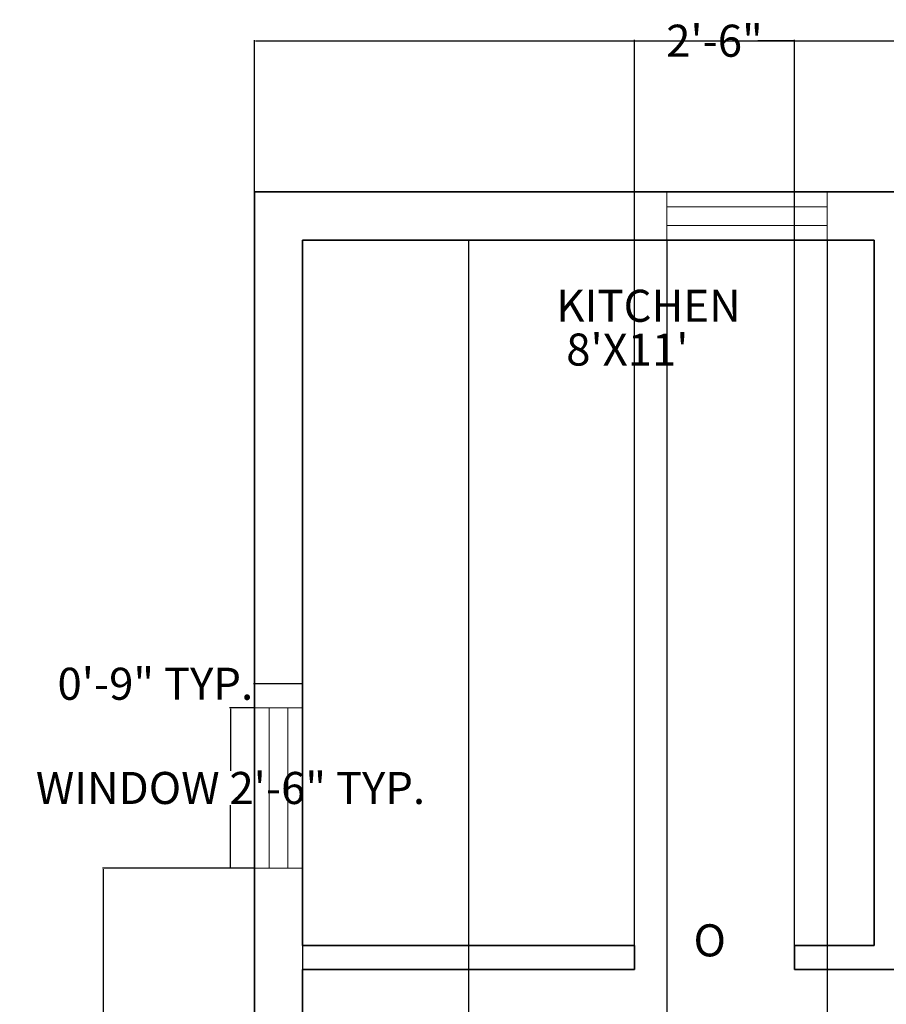
# Model space of a CAD drawing. Units: inches. Extents: x -26 to 575, y -18 to 513.
# Tile 10 of 28: x -26 to 136, y 324 to 508. Entities that reach past the tile are written whole.
import ezdxf

# ---------------------------------------------------------------- set-up
doc = ezdxf.new("R2010")
doc.units = ezdxf.units.IN
doc.header["$MEASUREMENT"] = 0
for name, color, linetype, lineweight in [('A-ANNO-DIMS', 2, 'Continuous', 18), ('A-ANNO-TEXT', 7, 'Continuous', 18), ('A-AREA-IDEN', 7, 'Continuous', 18), ('A-FLOR-CASE', 8, 'Continuous', 18), ('A-GLAZ', 4, 'Continuous', 18), ('A-WALL', 7, 'Continuous', 35)]:
    doc.layers.add(name, color=color, linetype=linetype, lineweight=lineweight)
doc.styles.get("Standard").update_dxf_attribs({"font": 'arial.ttf', "height": 6})
doc.dimstyles.get("Standard").update_dxf_attribs({"dimtxt": 6, "dimasz": 0.18, "dimexe": 0.18, "dimexo": 0.0625, "dimgap": 0.09, "dimtad": 0, "dimtih": 1, "dimtoh": 1, "dimzin": 0, "dimdsep": 46, "dimlunit": 3, "dimtxsty": 'Standard', "dimcen": 0.09, "dimadec": 0, "dimazin": 0, "dimtfac": 1, "dimtofl": 0, "dimtmove": 0, "dimatfit": 3, "dimfxl": 1, "dimtolj": 1, "dimtzin": 0, "dimarcsym": 0})

# ---------------------------------------------------------------- blocks, each defined once
blk = doc.blocks.new('*D1')
at = {"layer": 'A-ANNO-DIMS', "color": 0, "lineweight": -2, "transparency": 16777216}
for p, q in [((18.18, 475.57), (18.18, 503.94)), ((18.36, 503.76), (264.87, 503.76)), ((522, 503.76), (275.48, 503.76)), ((522.18, 475.57), (522.18, 503.94))]:
    blk.add_line(p, q, dxfattribs=at)
at = {"layer": 'A-ANNO-DIMS', "color": 0, "transparency": 16777216}
for points in [[(18.36, 503.79), (18.36, 503.73), (18.18, 503.76)], [(522, 503.79), (522, 503.73), (522.18, 503.76)]]:
    blk.add_solid(points, dxfattribs=at)
at = {"layer": 'Defpoints', "color": 0, "transparency": 16777216}
for p in [(522.18, 503.76), (18.18, 475.51), (522.18, 475.51)]:
    blk.add_point(p, dxfattribs=at)
at = {"layer": 'A-ANNO-DIMS', "color": 0, "transparency": 16777216, "insert": (270.18, 503.76), "char_height": 6, "attachment_point": 5}
blk.add_mtext("\\A1;42'", dxfattribs=at)
blk = doc.blocks.new('WINDOW-30IN')
for p, q in [((30, 9), (0, 9)), ((0, 9), (0, 0)), ((30, 0), (30, 9)), ((30, 6.25), (0, 6.25)), ((30, 0), (30, 4.5)), ((30, 2.75), (0, 2.75)), ((0, 0), (30, 0))]:
    blk.add_line(p, q)
blk = doc.blocks.new('*D18')
at = {"layer": 'A-ANNO-DIMS', "color": 0, "lineweight": -2, "transparency": 16777216}
for p, q in [((18.11, 378.99), (13.5, 378.99)), ((13.68, 378.81), (13.68, 367.18)), ((13.68, 349.17), (13.68, 360.79)), ((18.11, 348.99), (13.5, 348.99))]:
    blk.add_line(p, q, dxfattribs=at)
at = {"layer": 'A-ANNO-DIMS', "color": 0, "transparency": 16777216}
for points in [[(13.65, 378.81), (13.71, 378.81), (13.68, 378.99)], [(13.65, 349.17), (13.71, 349.17), (13.68, 348.99)]]:
    blk.add_solid(points, dxfattribs=at)
at = {"layer": 'Defpoints', "color": 0, "transparency": 16777216}
for p in [(18.18, 378.99), (13.68, 348.99), (18.18, 348.99)]:
    blk.add_point(p, dxfattribs=at)
at = {"layer": 'A-ANNO-DIMS', "color": 0, "transparency": 16777216, "insert": (13.68, 363.99), "char_height": 6, "attachment_point": 5}
blk.add_mtext('\\A1;WINDOW 2\'-6" TYP.', dxfattribs=at)
blk = doc.blocks.new('*D19')
at = {"layer": 'A-ANNO-DIMS', "color": 0, "lineweight": -2, "transparency": 16777216}
for p, q in [((18.18, 383.49), (18, 383.49)), ((18.18, 379.05), (18.18, 383.67)), ((27, 383.49), (18.36, 383.49)), ((27.18, 379.05), (27.18, 383.67))]:
    blk.add_line(p, q, dxfattribs=at)
at = {"layer": 'A-ANNO-DIMS', "color": 0, "transparency": 16777216}
for points in [[(18.36, 383.52), (18.36, 383.46), (18.18, 383.49)], [(27, 383.52), (27, 383.46), (27.18, 383.49)]]:
    blk.add_solid(points, dxfattribs=at)
at = {"layer": 'Defpoints', "color": 0, "transparency": 16777216}
for p in [(18.18, 383.49), (18.18, 378.99), (27.18, 378.99)]:
    blk.add_point(p, dxfattribs=at)
at = {"layer": 'A-ANNO-DIMS', "color": 0, "transparency": 16777216, "insert": (-0.38, 383.49), "char_height": 6, "attachment_point": 5}
blk.add_mtext('\\A1;0\'-9" TYP.', dxfattribs=at)
blk = doc.blocks.new('*D28')
at = {"layer": 'A-ANNO-DIMS', "color": 0, "lineweight": -2, "transparency": 16777216}
for p, q in [((58.22, 466.45), (58.22, -8.97)), ((95.35, 466.45), (95.35, -8.97)), ((58.4, -8.79), (68.72, -8.79)), ((95.17, -8.79), (84.85, -8.79))]:
    blk.add_line(p, q, dxfattribs=at)
at = {"layer": 'A-ANNO-DIMS', "color": 0, "transparency": 16777216}
for points in [[(58.4, -8.76), (58.4, -8.82), (58.22, -8.79)], [(95.17, -8.76), (95.17, -8.82), (95.35, -8.79)]]:
    blk.add_solid(points, dxfattribs=at)
at = {"layer": 'Defpoints', "color": 0, "transparency": 16777216}
for p in [(58.22, 466.51), (95.35, 466.51), (95.35, -8.79)]:
    blk.add_point(p, dxfattribs=at)
at = {"layer": 'A-ANNO-DIMS', "color": 0, "transparency": 16777216, "insert": (76.79, -8.79), "char_height": 6, "attachment_point": 5}
blk.add_mtext('\\A1;3\'-1"', dxfattribs=at)
blk = doc.blocks.new('*D29')
at = {"layer": 'A-ANNO-DIMS', "color": 0, "lineweight": -2, "transparency": 16777216}
for p, q in [((125.35, 466.45), (125.35, -8.97)), ((152.78, 466.45), (152.78, -8.97)), ((125.53, -8.79), (152.6, -8.79)), ((152.78, -8.79), (152.96, -8.79))]:
    blk.add_line(p, q, dxfattribs=at)
at = {"layer": 'A-ANNO-DIMS', "color": 0, "transparency": 16777216}
for points in [[(125.53, -8.76), (125.53, -8.82), (125.35, -8.79)], [(152.6, -8.76), (152.6, -8.82), (152.78, -8.79)]]:
    blk.add_solid(points, dxfattribs=at)
at = {"layer": 'Defpoints', "color": 0, "transparency": 16777216}
for p in [(125.35, 466.51), (152.78, 466.51), (152.78, -8.79)]:
    blk.add_point(p, dxfattribs=at)
at = {"layer": 'A-ANNO-DIMS', "color": 0, "transparency": 16777216, "insert": (168.07, -8.79), "char_height": 6, "attachment_point": 5}
blk.add_mtext('\\A1;2\'-3 1/2"', dxfattribs=at)
blk = doc.blocks.new('*D37')
at = {"layer": 'A-ANNO-DIMS', "color": 0, "lineweight": -2, "transparency": 16777216}
for p, q in [((18.11, 348.99), (-10.3, 348.99)), ((-10.12, 348.81), (-10.12, 311.43)), ((-10.12, 267.67), (-10.12, 305.05)), ((18.11, 267.49), (-10.3, 267.49))]:
    blk.add_line(p, q, dxfattribs=at)
at = {"layer": 'A-ANNO-DIMS', "color": 0, "transparency": 16777216}
for points in [[(-10.15, 348.81), (-10.09, 348.81), (-10.12, 348.99)], [(-10.15, 267.67), (-10.09, 267.67), (-10.12, 267.49)]]:
    blk.add_solid(points, dxfattribs=at)
at = {"layer": 'Defpoints', "color": 0, "transparency": 16777216}
for p in [(-10.12, 348.99), (18.18, 348.99), (18.18, 267.49)]:
    blk.add_point(p, dxfattribs=at)
at = {"layer": 'A-ANNO-DIMS', "color": 0, "transparency": 16777216, "insert": (-10.12, 308.24), "char_height": 6, "attachment_point": 5}
blk.add_mtext('\\A1;6\'-9 1/2"', dxfattribs=at)
blk = doc.blocks.new('*D46')
at = {"layer": 'A-ANNO-DIMS', "color": 0, "lineweight": -2, "transparency": 16777216}
for p, q in [((89.27, 334.57), (89.27, 503.99)), ((89.45, 503.81), (96.15, 503.81)), ((119.09, 503.81), (112.39, 503.81)), ((119.27, 334.57), (119.27, 503.99))]:
    blk.add_line(p, q, dxfattribs=at)
at = {"layer": 'A-ANNO-DIMS', "color": 0, "transparency": 16777216}
for points in [[(89.45, 503.84), (89.45, 503.78), (89.27, 503.81)], [(119.09, 503.84), (119.09, 503.78), (119.27, 503.81)]]:
    blk.add_solid(points, dxfattribs=at)
at = {"layer": 'Defpoints', "color": 0, "transparency": 16777216}
for p in [(119.27, 503.81), (89.27, 334.51), (119.27, 334.51)]:
    blk.add_point(p, dxfattribs=at)
at = {"layer": 'A-ANNO-DIMS', "color": 0, "transparency": 16777216, "insert": (104.27, 503.81), "char_height": 6, "attachment_point": 5}
blk.add_mtext('\\A1;2\'-6"', dxfattribs=at)
blk = doc.blocks.new('*D50')
at = {"layer": 'A-ANNO-DIMS', "color": 0, "lineweight": -2, "transparency": 16777216}
for p, q in [((27.18, 466.45), (27.18, -8.97)), ((58.22, 466.45), (58.22, -8.97)), ((27.36, -8.79), (34.58, -8.79)), ((58.04, -8.79), (50.82, -8.79))]:
    blk.add_line(p, q, dxfattribs=at)
at = {"layer": 'A-ANNO-DIMS', "color": 0, "transparency": 16777216}
for points in [[(27.36, -8.76), (27.36, -8.82), (27.18, -8.79)], [(58.04, -8.76), (58.04, -8.82), (58.22, -8.79)]]:
    blk.add_solid(points, dxfattribs=at)
at = {"layer": 'Defpoints', "color": 0, "transparency": 16777216}
for p in [(27.18, 466.51), (58.22, 466.51), (58.22, -8.79)]:
    blk.add_point(p, dxfattribs=at)
at = {"layer": 'A-ANNO-DIMS', "color": 0, "transparency": 16777216, "insert": (42.7, -8.79), "char_height": 6, "attachment_point": 5}
blk.add_mtext('\\A1;2\'-7"', dxfattribs=at)

msp = doc.modelspace()

# ---------------------------------------------------------------- linework, layer by layer
at = {"layer": 'A-FLOR-CASE'}
msp.add_line((58.224, 334.508), (58.224, 466.508), dxfattribs=at)
at = {"layer": 'A-WALL'}
for p, q in [((27.177, 466.508), (27.177, 334.508)), ((134.177, 466.508), (27.177, 466.508)), ((134.177, 334.508), (134.177, 466.508)), ((89.27, 334.508), (27.177, 334.508)), ((89.27, 334.508), (89.27, 330.008)), ((134.177, 334.508), (119.27, 334.508)), ((119.27, 334.508), (119.27, 330.008)), ((27.177, 330.008), (27.177, 127.508)), ((89.27, 330.008), (27.177, 330.008)), ((134.177, 330.008), (119.27, 330.008)), ((147.498, 330.008), (134.177, 330.008))]:
    msp.add_line(p, q, dxfattribs=at)
msp.add_lwpolyline([(18.177, 19.508), (522.177, 19.508), (522.177, 475.508), (18.177, 475.508)], close=True, dxfattribs=at)

# ---------------------------------------------------------------- block references
at = {"layer": 'A-GLAZ'}
msp.add_blockref('WINDOW-30IN', (95.349, 466.508), dxfattribs=at)
at = {"layer": 'A-GLAZ', "extrusion": (0, 0, -1), "zscale": -1, "rotation": 270.0000000000003}
msp.add_blockref('WINDOW-30IN', (-27.177, 378.988), dxfattribs=at)

# ---------------------------------------------------------------- texts
at = {"layer": 'A-ANNO-TEXT'}
msp.add_text('O', height=6, rotation=0.00167, dxfattribs=at).set_placement((100.345, 332.476))
at = {"layer": 'A-AREA-IDEN'}
for s, p in [('KITCHEN', (74.673, 451.211)), ("8'X11'", (76.522, 443.024))]:
    msp.add_text(s, height=6, rotation=0.00167, dxfattribs=at).set_placement(p)

# ---------------------------------------------------------------- dimensions: what is measured, and where the dimension line sits
at = {"layer": 'A-ANNO-DIMS'}
for base, p1, p2, override, picture, middle in [((522.177, 503.757), (18.177, 475.508), (522.177, 475.508), {"dimclrd": 0, "dimclre": 0, "dimclrt": 0}, '*D1', (270.177, 503.757)), ((119.27, 503.808), (89.27, 334.508), (119.27, 334.508), {"dimdec": 1, "dimlfac": 1, "dimrnd": 0, "dimzin": 1, "dimdsep": 46, "dimlunit": 4, "dimfrac": 2}, '*D46', (104.27, 503.808)), ((58.224, -8.792), (27.177, 466.508), (58.224, 466.508), {"dimdec": 1, "dimlfac": 1, "dimrnd": 0, "dimzin": 1, "dimdsep": 46, "dimlunit": 4, "dimfrac": 2}, '*D50', (42.7, -8.792)), ((95.349, -8.792), (58.224, 466.508), (95.349, 466.508), {"dimdec": 1, "dimlfac": 1, "dimrnd": 0, "dimzin": 1, "dimdsep": 46, "dimlunit": 4, "dimfrac": 2}, '*D28', (76.786, -8.792)), ((152.784, -8.792), (125.349, 466.508), (152.784, 466.508), {"dimdec": 1, "dimlfac": 1, "dimrnd": 0, "dimzin": 1, "dimdsep": 46, "dimlunit": 4, "dimfrac": 2}, '*D29', (168.07, -8.792))]:
    dim = msp.add_linear_dim(base=base, p1=p1, p2=p2, dimstyle='Standard', override=override, dxfattribs=at)
    dim.commit()
    dim.dimension.update_dxf_attribs({"geometry": picture, "text_midpoint": middle})
for base, p1, p2, angle, text, picture, middle in [((18.177, 383.488), (27.177, 378.988), (18.177, 378.988), 180, '<> TYP.', '*D19', (-0.379, 383.488)), ((13.677, 348.988), (18.177, 378.988), (18.177, 348.988), 270, 'WINDOW <> TYP.', '*D18', (13.677, 363.988))]:
    dim = msp.add_linear_dim(base=base, p1=p1, p2=p2, angle=angle, text=text, dimstyle='Standard', override={"dimdec": 1, "dimlfac": 1, "dimrnd": 0, "dimzin": 1, "dimdsep": 46, "dimlunit": 4, "dimfrac": 2}, dxfattribs=at)
    dim.commit()
    dim.dimension.update_dxf_attribs({"geometry": picture, "text_midpoint": middle})
dim = msp.add_linear_dim(base=(-10.123, 348.988), p1=(18.177, 267.494), p2=(18.177, 348.988), angle=90, dimstyle='Standard', override={"dimdec": 1, "dimlfac": 1, "dimrnd": 0, "dimzin": 1, "dimdsep": 46, "dimlunit": 4, "dimfrac": 2}, dxfattribs=at)
dim.commit()
dim.dimension.update_dxf_attribs({"geometry": '*D37', "text_midpoint": (-10.123, 308.241)})

doc.saveas('drawing.dxf')
